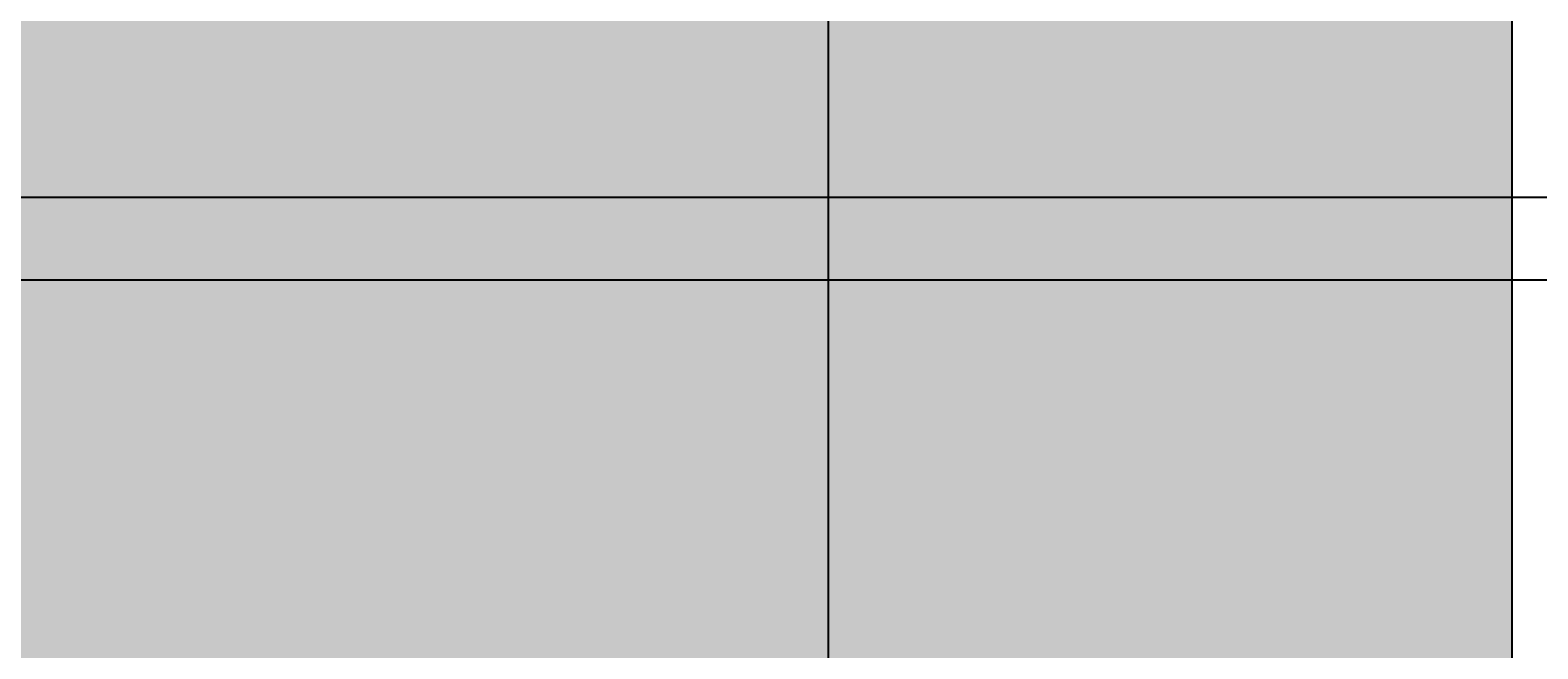
# Model space of a CAD drawing. Units: inches. Extents: x 35362 to 73946, y 43607 to 67532.
# Tile 65 of 134: x 47763 to 48170, y 48798 to 48965. Entities that reach past the tile are written whole.
import ezdxf

# ---------------------------------------------------------------- set-up
doc = ezdxf.new("R2010")
doc.units = ezdxf.units.IN
doc.header["$MEASUREMENT"] = 0
for name, color, linetype, lineweight in [('A-ANNO-DIMS', 2, 'Continuous', 18), ('E-SYMB', 1, 'Continuous', 25), ('E-SYMB-PATT', 1, 'Continuous', 13)]:
    doc.layers.add(name, color=color, linetype=linetype, lineweight=lineweight)
doc.styles.get("Standard").update_dxf_attribs({"font": 'arial.ttf'})
doc.dimstyles.get("Standard").update_dxf_attribs({"dimtxt": 0.18, "dimasz": 0.18, "dimexe": 0.18, "dimexo": 0.0625, "dimgap": 0.09, "dimtad": 0, "dimtih": 1, "dimtoh": 1, "dimdec": 4, "dimzin": 0, "dimdsep": 46, "dimtxsty": 'Standard', "dimcen": 0.09, "dimadec": 0, "dimazin": 0, "dimtfac": 1, "dimtdec": 4, "dimtofl": 0, "dimtmove": 0, "dimatfit": 3, "dimfxl": 1, "dimtolj": 1, "dimtzin": 0, "dimarcsym": 0})

# ---------------------------------------------------------------- blocks, each defined once
blk = doc.blocks.new('*D11')
at = {"layer": 'A-ANNO-DIMS', "color": 0, "lineweight": -2, "transparency": 16777216}
for p, q in [((47978.66, 56028.77), (47978.66, 43606.68)), ((53109.76, 56028.77), (53109.76, 43606.68)), ((47978.84, 43606.86), (50543.87, 43606.86)), ((53109.58, 43606.86), (50544.55, 43606.86))]:
    blk.add_line(p, q, dxfattribs=at)
at = {"layer": 'A-ANNO-DIMS', "color": 0, "transparency": 16777216}
for points in [[(47978.84, 43606.89), (47978.84, 43606.83), (47978.66, 43606.86)], [(53109.58, 43606.89), (53109.58, 43606.83), (53109.76, 43606.86)]]:
    blk.add_solid(points, dxfattribs=at)
at = {"layer": 'Defpoints', "color": 0, "transparency": 16777216}
for p in [(47978.66, 56028.84), (53109.76, 56028.84), (53109.76, 43606.86)]:
    blk.add_point(p, dxfattribs=at)
at = {"layer": 'A-ANNO-DIMS', "color": 0, "transparency": 16777216, "insert": (50544.21, 43606.86), "char_height": 0.18, "attachment_point": 5}
blk.add_mtext('\\A1;5131', dxfattribs=at)
blk = doc.blocks.new('*D27')
at = {"layer": 'A-ANNO-DIMS', "color": 0, "lineweight": -2, "transparency": 16777216}
for p, q in [((47978.66, 56028.77), (47978.66, 43606.68)), ((48373.49, 53428.96), (48373.49, 43606.68)), ((47978.84, 43606.86), (48175.68, 43606.86)), ((48373.31, 43606.86), (48176.47, 43606.86))]:
    blk.add_line(p, q, dxfattribs=at)
at = {"layer": 'A-ANNO-DIMS', "color": 0, "transparency": 16777216}
for points in [[(47978.84, 43606.89), (47978.84, 43606.83), (47978.66, 43606.86)], [(48373.31, 43606.89), (48373.31, 43606.83), (48373.49, 43606.86)]]:
    blk.add_solid(points, dxfattribs=at)
at = {"layer": 'Defpoints', "color": 0, "transparency": 16777216}
for p in [(47978.66, 56028.84), (48373.49, 53429.02), (48373.49, 43606.86)]:
    blk.add_point(p, dxfattribs=at)
at = {"layer": 'A-ANNO-DIMS', "color": 0, "transparency": 16777216, "insert": (48176.08, 43606.86), "char_height": 0.18, "attachment_point": 5}
blk.add_mtext('\\A1;394.8', dxfattribs=at)
blk = doc.blocks.new('*D67')
at = {"layer": 'A-ANNO-DIMS', "color": 0, "lineweight": -2, "transparency": 16777216}
for p, q in [((56873.54, 53351.53), (35361.77, 53351.53)), ((35361.95, 53351.35), (35361.95, 49400.89)), ((35361.95, 45450.07), (35361.95, 49400.53)), ((53793.58, 45449.89), (35361.77, 45449.89))]:
    blk.add_line(p, q, dxfattribs=at)
at = {"layer": 'A-ANNO-DIMS', "color": 0, "transparency": 16777216}
for points in [[(35361.92, 53351.35), (35361.98, 53351.35), (35361.95, 53351.53)], [(35361.92, 45450.07), (35361.98, 45450.07), (35361.95, 45449.89)]]:
    blk.add_solid(points, dxfattribs=at)
at = {"layer": 'Defpoints', "color": 0, "transparency": 16777216}
for p in [(35361.95, 53351.53), (56873.6, 53351.53), (53793.64, 45449.89)]:
    blk.add_point(p, dxfattribs=at)
at = {"layer": 'A-ANNO-DIMS', "color": 0, "transparency": 16777216, "insert": (35361.95, 49400.71), "char_height": 0.18, "attachment_point": 5}
blk.add_mtext('\\A1;7901.6', dxfattribs=at)
blk = doc.blocks.new('*D86')
at = {"layer": 'A-ANNO-DIMS', "color": 0, "lineweight": -2, "transparency": 16777216}
for p, q in [((51285.53, 49320.08), (35361.77, 49320.08)), ((35361.95, 49319.9), (35361.95, 49120.26)), ((35361.95, 48920.26), (35361.95, 49119.9)), ((51285.53, 48920.08), (35361.77, 48920.08))]:
    blk.add_line(p, q, dxfattribs=at)
at = {"layer": 'A-ANNO-DIMS', "color": 0, "transparency": 16777216}
for points in [[(35361.92, 49319.9), (35361.98, 49319.9), (35361.95, 49320.08)], [(35361.92, 48920.26), (35361.98, 48920.26), (35361.95, 48920.08)]]:
    blk.add_solid(points, dxfattribs=at)
at = {"layer": 'Defpoints', "color": 0, "transparency": 16777216}
for p in [(35361.95, 49320.08), (51285.59, 49320.08), (51285.59, 48920.08)]:
    blk.add_point(p, dxfattribs=at)
at = {"layer": 'A-ANNO-DIMS', "color": 0, "transparency": 16777216, "insert": (35361.95, 49120.08), "char_height": 0.18, "attachment_point": 5}
blk.add_mtext('\\A1;400.0', dxfattribs=at)
blk = doc.blocks.new('*D89')
at = {"layer": 'A-ANNO-DIMS', "color": 0, "lineweight": -2, "transparency": 16777216}
for p, q in [((53707.72, 48897.74), (35361.77, 48897.74)), ((35361.95, 48897.56), (35361.95, 48303.16)), ((35361.95, 47708.4), (35361.95, 48302.8)), ((53707.72, 47708.22), (35361.77, 47708.22))]:
    blk.add_line(p, q, dxfattribs=at)
at = {"layer": 'A-ANNO-DIMS', "color": 0, "transparency": 16777216}
for points in [[(35361.92, 48897.56), (35361.98, 48897.56), (35361.95, 48897.74)], [(35361.92, 47708.4), (35361.98, 47708.4), (35361.95, 47708.22)]]:
    blk.add_solid(points, dxfattribs=at)
at = {"layer": 'Defpoints', "color": 0, "transparency": 16777216}
for p in [(53707.78, 48897.74), (35361.95, 47708.22), (53707.78, 47708.22)]:
    blk.add_point(p, dxfattribs=at)
at = {"layer": 'A-ANNO-DIMS', "color": 0, "transparency": 16777216, "insert": (35361.95, 48302.98), "char_height": 0.18, "attachment_point": 5}
blk.add_mtext('\\A1;1189.5', dxfattribs=at)

msp = doc.modelspace()

# ---------------------------------------------------------------- hatches: boundary and pattern name
at = {"layer": 'E-SYMB-PATT'}
h = msp.add_hatch(color=256, dxfattribs=at)
h.dxf.hatch_style = 1
h.paths.add_polyline_path([(48163.038, 49689.843), (45390.147, 49689.843), (45390.147, 46919.381), (48163.038, 46919.381)])

# ---------------------------------------------------------------- linework, layer by layer
at = {"layer": 'E-SYMB'}
msp.add_lwpolyline([(45390.147, 49689.843), (48163.038, 49689.843), (48163.038, 46919.381), (45390.147, 46919.381)], close=True, dxfattribs=at)

# ---------------------------------------------------------------- dimensions: what is measured, and where the dimension line sits
at = {"layer": 'A-ANNO-DIMS'}
for base, p2, override, picture, middle in [((53109.76, 43606.859), (53109.76, 56028.836), {"dimdec": 0, "dimlfac": 1, "dimrnd": 0, "dimzin": 0, "dimdsep": 46, "dimlunit": 2}, '*D11', (50544.212, 43606.859)), ((48373.492, 43606.859), (48373.492, 53429.019), {"dimdec": 1, "dimlfac": 1, "dimrnd": 0, "dimzin": 0, "dimdsep": 46, "dimlunit": 2}, '*D27', (48176.078, 43606.859))]:
    dim = msp.add_linear_dim(base=base, p1=(47978.665, 56028.836), p2=p2, dimstyle='Standard', override=override, dxfattribs=at)
    dim.commit()
    dim.dimension.update_dxf_attribs({"geometry": picture, "text_midpoint": middle})
for base, p1, p2, picture, middle in [((35361.949, 53351.529), (53793.638, 45449.894), (56873.602, 53351.529), '*D67', (35361.949, 49400.712)), ((35361.949, 49320.079), (51285.595, 48920.079), (51285.595, 49320.079), '*D86', (35361.949, 49120.079)), ((35361.949, 47708.216), (53707.781, 48897.738), (53707.781, 47708.216), '*D89', (35361.949, 48302.977))]:
    dim = msp.add_linear_dim(base=base, p1=p1, p2=p2, angle=90, dimstyle='Standard', override={"dimdec": 1, "dimlfac": 1, "dimrnd": 0, "dimzin": 0, "dimdsep": 46, "dimlunit": 2}, dxfattribs=at)
    dim.commit()
    dim.dimension.update_dxf_attribs({"geometry": picture, "text_midpoint": middle})

doc.saveas('drawing.dxf')
